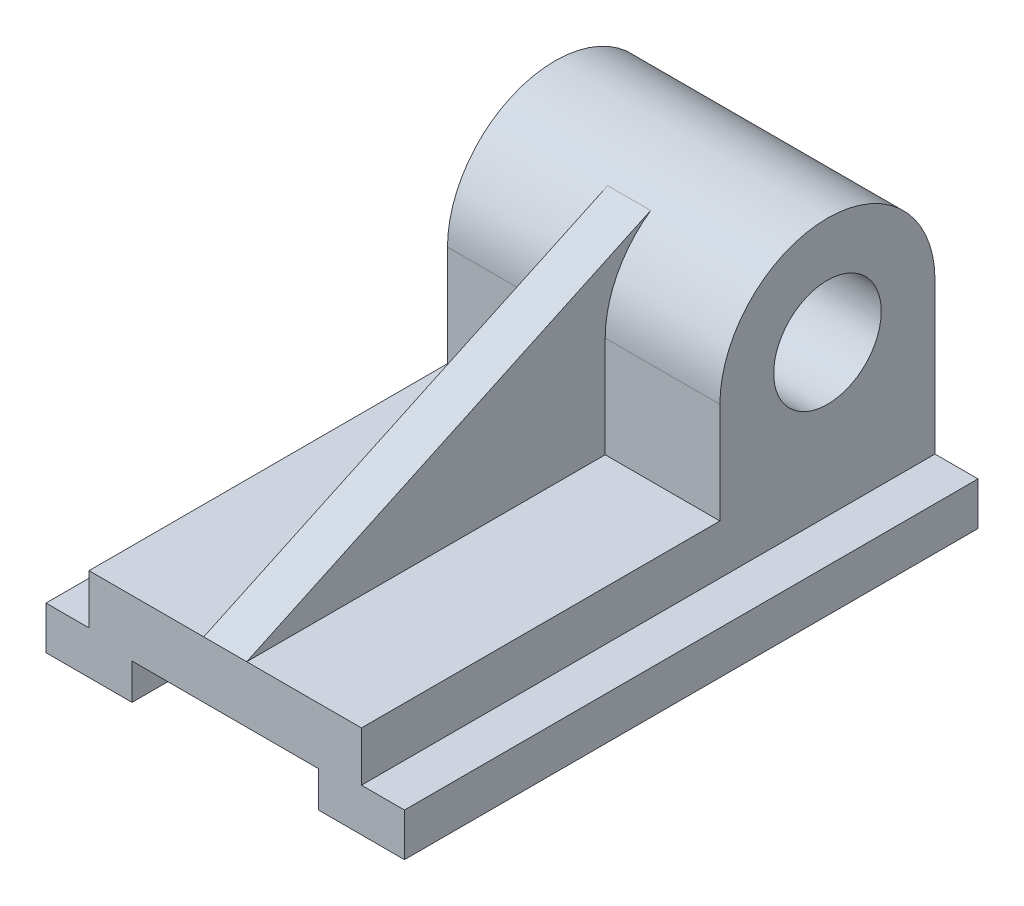
ISO-10303-21;
HEADER;
FILE_DESCRIPTION(('STEP AP214'),'2;1');
FILE_NAME('part.step','',(''),(''),'','','');
FILE_SCHEMA(('AUTOMOTIVE_DESIGN { 1 0 10303 214 1 1 1 1 }'));
ENDSEC;
DATA;
#1=APPLICATION_CONTEXT('core data for automotive mechanical design processes');
#2=APPLICATION_PROTOCOL_DEFINITION('international standard','automotive_design',2000,#1);
#3=PRODUCT_CONTEXT('',#1,'mechanical');
#4=PRODUCT('Part','Part','',(#3));
#5=PRODUCT_RELATED_PRODUCT_CATEGORY('part','',(#4));
#6=PRODUCT_DEFINITION_FORMATION('','',#4);
#7=PRODUCT_DEFINITION_CONTEXT('part definition',#1,'design');
#8=PRODUCT_DEFINITION('design','',#6,#7);
#9=PRODUCT_DEFINITION_SHAPE('','',#8);
#10=(LENGTH_UNIT() NAMED_UNIT(*) SI_UNIT(.MILLI.,.METRE.));
#11=(NAMED_UNIT(*) PLANE_ANGLE_UNIT() SI_UNIT($,.RADIAN.));
#12=(NAMED_UNIT(*) SI_UNIT($,.STERADIAN.) SOLID_ANGLE_UNIT());
#13=UNCERTAINTY_MEASURE_WITH_UNIT(LENGTH_MEASURE(1.E-05),#10,'distance_accuracy_value','');
#14=(GEOMETRIC_REPRESENTATION_CONTEXT(3) GLOBAL_UNCERTAINTY_ASSIGNED_CONTEXT((#13)) GLOBAL_UNIT_ASSIGNED_CONTEXT((#10,
#11,#12)) REPRESENTATION_CONTEXT('',''));
#15=CARTESIAN_POINT('',(0.,0.,0.));
#16=DIRECTION('',(0.,0.,1.));
#17=DIRECTION('',(1.,0.,0.));
#18=AXIS2_PLACEMENT_3D('',#15,#16,#17);
#19=CARTESIAN_POINT('',(-50.,44.,30.));
#20=DIRECTION('',(1.,0.,0.));
#21=DIRECTION('',(0.,0.,-1.));
#22=AXIS2_PLACEMENT_3D('',#19,#20,#21);
#23=CYLINDRICAL_SURFACE('',#22,30.);
#24=DIRECTION('',(-1.,0.,0.));
#25=VECTOR('',#24,1.);
#26=CARTESIAN_POINT('',(6.,68.5011775972043,47.3116231575856));
#27=LINE('',#26,#25);
#28=CARTESIAN_POINT('',(6.,68.5011775972043,47.3116231575856));
#29=VERTEX_POINT('',#28);
#30=CARTESIAN_POINT('',(-6.,68.5011775972043,47.3116231575856));
#31=VERTEX_POINT('',#30);
#32=EDGE_CURVE('E324',#29,#31,#27,.T.);
#33=ORIENTED_EDGE('',*,*,#32,.F.);
#34=CARTESIAN_POINT('',(6.,43.9999999999999,29.9999999999998));
#35=DIRECTION('',(-1.,0.,0.));
#36=DIRECTION('',(0.,0.,1.));
#37=AXIS2_PLACEMENT_3D('',#34,#35,#36);
#38=CIRCLE('',#37,30.0000000000002);
#39=CARTESIAN_POINT('',(6.,44.,60.));
#40=VERTEX_POINT('',#39);
#41=EDGE_CURVE('E191',#40,#29,#38,.T.);
#42=ORIENTED_EDGE('',*,*,#41,.F.);
#43=DIRECTION('',(1.,0.,0.));
#44=VECTOR('',#43,1.);
#45=CARTESIAN_POINT('',(-50.,44.,60.));
#46=LINE('',#45,#44);
#47=CARTESIAN_POINT('',(38.,44.,60.));
#48=VERTEX_POINT('',#47);
#49=EDGE_CURVE('E188',#40,#48,#46,.T.);
#50=ORIENTED_EDGE('',*,*,#49,.T.);
#51=CARTESIAN_POINT('',(38.,44.,30.));
#52=DIRECTION('',(1.,0.,0.));
#53=DIRECTION('',(0.,0.,-1.));
#54=AXIS2_PLACEMENT_3D('',#51,#52,#53);
#55=CIRCLE('',#54,30.);
#56=CARTESIAN_POINT('',(38.,44.,0.));
#57=VERTEX_POINT('',#56);
#58=EDGE_CURVE('E302',#57,#48,#55,.T.);
#59=ORIENTED_EDGE('',*,*,#58,.F.);
#60=DIRECTION('',(1.,0.,0.));
#61=VECTOR('',#60,1.);
#62=CARTESIAN_POINT('',(-50.,44.,0.));
#63=LINE('',#62,#61);
#64=CARTESIAN_POINT('',(-38.,44.,0.));
#65=VERTEX_POINT('',#64);
#66=EDGE_CURVE('E11',#65,#57,#63,.T.);
#67=ORIENTED_EDGE('',*,*,#66,.F.);
#68=CARTESIAN_POINT('',(-38.,44.,30.));
#69=DIRECTION('',(-1.,0.,0.));
#70=DIRECTION('',(0.,0.,1.));
#71=AXIS2_PLACEMENT_3D('',#68,#69,#70);
#72=CIRCLE('',#71,30.);
#73=CARTESIAN_POINT('',(-38.,44.,60.));
#74=VERTEX_POINT('',#73);
#75=EDGE_CURVE('E55',#74,#65,#72,.T.);
#76=ORIENTED_EDGE('',*,*,#75,.F.);
#77=CARTESIAN_POINT('',(-6.,44.,60.));
#78=VERTEX_POINT('',#77);
#79=EDGE_CURVE('E204',#74,#78,#46,.T.);
#80=ORIENTED_EDGE('',*,*,#79,.T.);
#81=CARTESIAN_POINT('',(-6.,43.9999999999999,29.9999999999998));
#82=DIRECTION('',(-1.,0.,0.));
#83=DIRECTION('',(0.,0.,1.));
#84=AXIS2_PLACEMENT_3D('',#81,#82,#83);
#85=CIRCLE('',#84,30.0000000000002);
#86=EDGE_CURVE('E335',#78,#31,#85,.T.);
#87=ORIENTED_EDGE('',*,*,#86,.T.);
#88=EDGE_LOOP('',(#33,#42,#50,#59,#67,#76,#80,#87));
#89=FACE_BOUND('',#88,.T.);
#90=ADVANCED_FACE('F43',(#89),#23,.T.);
#91=CARTESIAN_POINT('',(-50.,0.,60.));
#92=DIRECTION('',(0.,0.,1.));
#93=DIRECTION('',(1.,0.,0.));
#94=AXIS2_PLACEMENT_3D('',#91,#92,#93);
#95=PLANE('',#94);
#96=ORIENTED_EDGE('',*,*,#49,.F.);
#97=DIRECTION('',(0.,1.,0.));
#98=VECTOR('',#97,1.);
#99=CARTESIAN_POINT('',(6.,15.8288601385803,60.));
#100=LINE('',#99,#98);
#101=CARTESIAN_POINT('',(6.,15.8288601385803,60.));
#102=VERTEX_POINT('',#101);
#103=EDGE_CURVE('E171',#102,#40,#100,.T.);
#104=ORIENTED_EDGE('',*,*,#103,.F.);
#105=DIRECTION('',(1.,0.,0.));
#106=VECTOR('',#105,1.);
#107=CARTESIAN_POINT('',(-50.,15.8288601385803,60.));
#108=LINE('',#107,#106);
#109=CARTESIAN_POINT('',(38.,15.8288601385803,60.));
#110=VERTEX_POINT('',#109);
#111=EDGE_CURVE('E190',#102,#110,#108,.T.);
#112=ORIENTED_EDGE('',*,*,#111,.T.);
#113=DIRECTION('',(0.,-1.,0.));
#114=VECTOR('',#113,1.);
#115=CARTESIAN_POINT('',(38.,0.,60.));
#116=LINE('',#115,#114);
#117=EDGE_CURVE('E196',#48,#110,#116,.T.);
#118=ORIENTED_EDGE('',*,*,#117,.F.);
#119=EDGE_LOOP('',(#96,#104,#112,#118));
#120=FACE_BOUND('',#119,.T.);
#121=ADVANCED_FACE('F187',(#120),#95,.T.);
#122=CARTESIAN_POINT('',(-50.,15.8288601385803,0.));
#123=DIRECTION('',(0.,-1.,0.));
#124=DIRECTION('',(0.,0.,-1.));
#125=AXIS2_PLACEMENT_3D('',#122,#123,#124);
#126=PLANE('',#125);
#127=DIRECTION('',(0.,0.,-1.));
#128=VECTOR('',#127,1.);
#129=CARTESIAN_POINT('',(6.,15.8288601385803,160.));
#130=LINE('',#129,#128);
#131=CARTESIAN_POINT('',(6.,15.8288601385803,160.));
#132=VERTEX_POINT('',#131);
#133=EDGE_CURVE('E172',#132,#102,#130,.T.);
#134=ORIENTED_EDGE('',*,*,#133,.F.);
#135=DIRECTION('',(1.,0.,0.));
#136=VECTOR('',#135,1.);
#137=CARTESIAN_POINT('',(0.,15.8288601385803,160.));
#138=LINE('',#137,#136);
#139=CARTESIAN_POINT('',(38.,15.8288601385803,160.));
#140=VERTEX_POINT('',#139);
#141=EDGE_CURVE('E287',#132,#140,#138,.T.);
#142=ORIENTED_EDGE('',*,*,#141,.T.);
#143=DIRECTION('',(0.,0.,-1.));
#144=VECTOR('',#143,1.);
#145=CARTESIAN_POINT('',(38.,15.8288601385803,0.));
#146=LINE('',#145,#144);
#147=EDGE_CURVE('E195',#140,#110,#146,.T.);
#148=ORIENTED_EDGE('',*,*,#147,.T.);
#149=ORIENTED_EDGE('',*,*,#111,.F.);
#150=EDGE_LOOP('',(#134,#142,#148,#149));
#151=FACE_BOUND('',#150,.T.);
#152=ADVANCED_FACE('F194',(#151),#126,.F.);
#153=CARTESIAN_POINT('',(38.,0.,160.));
#154=DIRECTION('',(-1.,0.,0.));
#155=DIRECTION('',(0.,0.,1.));
#156=AXIS2_PLACEMENT_3D('',#153,#154,#155);
#157=PLANE('',#156);
#158=CARTESIAN_POINT('',(38.,44.,30.));
#159=DIRECTION('',(1.,0.,0.));
#160=DIRECTION('',(0.,0.,-1.));
#161=AXIS2_PLACEMENT_3D('',#158,#159,#160);
#162=CIRCLE('',#161,15.);
#163=CARTESIAN_POINT('',(38.,44.,15.));
#164=VERTEX_POINT('',#163);
#165=EDGE_CURVE('E339',#164,#164,#162,.T.);
#166=ORIENTED_EDGE('',*,*,#165,.F.);
#167=EDGE_LOOP('',(#166));
#168=FACE_BOUND('',#167,.T.);
#169=DIRECTION('',(0.,1.,0.));
#170=VECTOR('',#169,1.);
#171=CARTESIAN_POINT('',(38.,0.,0.));
#172=LINE('',#171,#170);
#173=CARTESIAN_POINT('',(38.,2.,0.));
#174=VERTEX_POINT('',#173);
#175=EDGE_CURVE('E206',#174,#57,#172,.T.);
#176=ORIENTED_EDGE('',*,*,#175,.T.);
#177=ORIENTED_EDGE('',*,*,#58,.T.);
#178=ORIENTED_EDGE('',*,*,#117,.T.);
#179=ORIENTED_EDGE('',*,*,#147,.F.);
#180=DIRECTION('',(0.,1.,0.));
#181=VECTOR('',#180,1.);
#182=CARTESIAN_POINT('',(38.,0.,160.));
#183=LINE('',#182,#181);
#184=CARTESIAN_POINT('',(38.,2.,160.));
#185=VERTEX_POINT('',#184);
#186=EDGE_CURVE('E210',#185,#140,#183,.T.);
#187=ORIENTED_EDGE('',*,*,#186,.F.);
#188=DIRECTION('',(0.,0.,-1.));
#189=VECTOR('',#188,1.);
#190=CARTESIAN_POINT('',(38.,2.,160.));
#191=LINE('',#190,#189);
#192=EDGE_CURVE('E237',#185,#174,#191,.T.);
#193=ORIENTED_EDGE('',*,*,#192,.T.);
#194=EDGE_LOOP('',(#176,#177,#178,#179,#187,#193));
#195=FACE_BOUND('',#194,.T.);
#196=ADVANCED_FACE('F44',(#168,#195),#157,.F.);
#197=CARTESIAN_POINT('',(-38.,0.,160.));
#198=DIRECTION('',(-1.,0.,0.));
#199=DIRECTION('',(0.,0.,1.));
#200=AXIS2_PLACEMENT_3D('',#197,#198,#199);
#201=PLANE('',#200);
#202=CARTESIAN_POINT('',(-38.,44.,30.));
#203=DIRECTION('',(-1.,0.,0.));
#204=DIRECTION('',(0.,0.,1.));
#205=AXIS2_PLACEMENT_3D('',#202,#203,#204);
#206=CIRCLE('',#205,15.);
#207=CARTESIAN_POINT('',(-38.,44.,45.));
#208=VERTEX_POINT('',#207);
#209=EDGE_CURVE('E50',#208,#208,#206,.T.);
#210=ORIENTED_EDGE('',*,*,#209,.F.);
#211=EDGE_LOOP('',(#210));
#212=FACE_BOUND('',#211,.T.);
#213=ORIENTED_EDGE('',*,*,#75,.T.);
#214=DIRECTION('',(0.,1.,0.));
#215=VECTOR('',#214,1.);
#216=CARTESIAN_POINT('',(-38.,0.,0.));
#217=LINE('',#216,#215);
#218=CARTESIAN_POINT('',(-38.,2.,0.));
#219=VERTEX_POINT('',#218);
#220=EDGE_CURVE('E239',#219,#65,#217,.T.);
#221=ORIENTED_EDGE('',*,*,#220,.F.);
#222=DIRECTION('',(0.,0.,-1.));
#223=VECTOR('',#222,1.);
#224=CARTESIAN_POINT('',(-38.,2.,160.));
#225=LINE('',#224,#223);
#226=CARTESIAN_POINT('',(-38.,2.,160.));
#227=VERTEX_POINT('',#226);
#228=EDGE_CURVE('E283',#227,#219,#225,.T.);
#229=ORIENTED_EDGE('',*,*,#228,.F.);
#230=DIRECTION('',(0.,1.,0.));
#231=VECTOR('',#230,1.);
#232=CARTESIAN_POINT('',(-38.,0.,160.));
#233=LINE('',#232,#231);
#234=CARTESIAN_POINT('',(-38.,15.8288601385803,160.));
#235=VERTEX_POINT('',#234);
#236=EDGE_CURVE('E209',#227,#235,#233,.T.);
#237=ORIENTED_EDGE('',*,*,#236,.T.);
#238=DIRECTION('',(0.,0.,1.));
#239=VECTOR('',#238,1.);
#240=CARTESIAN_POINT('',(-38.,15.8288601385803,160.));
#241=LINE('',#240,#239);
#242=CARTESIAN_POINT('',(-38.,15.8288601385803,60.));
#243=VERTEX_POINT('',#242);
#244=EDGE_CURVE('E67',#243,#235,#241,.T.);
#245=ORIENTED_EDGE('',*,*,#244,.F.);
#246=DIRECTION('',(0.,1.,0.));
#247=VECTOR('',#246,1.);
#248=CARTESIAN_POINT('',(-38.,0.,60.));
#249=LINE('',#248,#247);
#250=EDGE_CURVE('E290',#243,#74,#249,.T.);
#251=ORIENTED_EDGE('',*,*,#250,.T.);
#252=EDGE_LOOP('',(#213,#221,#229,#237,#245,#251));
#253=FACE_BOUND('',#252,.T.);
#254=ADVANCED_FACE('F297',(#212,#253),#201,.T.);
#255=CARTESIAN_POINT('',(0.,2.,160.));
#256=DIRECTION('',(0.,1.,0.));
#257=DIRECTION('',(0.,0.,1.));
#258=AXIS2_PLACEMENT_3D('',#255,#256,#257);
#259=PLANE('',#258);
#260=DIRECTION('',(1.,0.,0.));
#261=VECTOR('',#260,1.);
#262=CARTESIAN_POINT('',(0.,2.,0.));
#263=LINE('',#262,#261);
#264=CARTESIAN_POINT('',(-50.,2.,0.));
#265=VERTEX_POINT('',#264);
#266=EDGE_CURVE('E244',#265,#219,#263,.T.);
#267=ORIENTED_EDGE('',*,*,#266,.F.);
#268=DIRECTION('',(0.,0.,-1.));
#269=VECTOR('',#268,1.);
#270=CARTESIAN_POINT('',(-50.,2.,160.));
#271=LINE('',#270,#269);
#272=CARTESIAN_POINT('',(-50.,2.,160.));
#273=VERTEX_POINT('',#272);
#274=EDGE_CURVE('E285',#273,#265,#271,.T.);
#275=ORIENTED_EDGE('',*,*,#274,.F.);
#276=DIRECTION('',(1.,0.,0.));
#277=VECTOR('',#276,1.);
#278=CARTESIAN_POINT('',(0.,2.,160.));
#279=LINE('',#278,#277);
#280=EDGE_CURVE('E212',#273,#227,#279,.T.);
#281=ORIENTED_EDGE('',*,*,#280,.T.);
#282=ORIENTED_EDGE('',*,*,#228,.T.);
#283=EDGE_LOOP('',(#267,#275,#281,#282));
#284=FACE_BOUND('',#283,.T.);
#285=ADVANCED_FACE('F310',(#284),#259,.T.);
#286=CARTESIAN_POINT('',(-50.,0.,160.));
#287=DIRECTION('',(-1.,0.,0.));
#288=DIRECTION('',(0.,0.,1.));
#289=AXIS2_PLACEMENT_3D('',#286,#287,#288);
#290=PLANE('',#289);
#291=DIRECTION('',(0.,1.,0.));
#292=VECTOR('',#291,1.);
#293=CARTESIAN_POINT('',(-50.,0.,0.));
#294=LINE('',#293,#292);
#295=CARTESIAN_POINT('',(-50.,-10.,0.));
#296=VERTEX_POINT('',#295);
#297=EDGE_CURVE('E243',#296,#265,#294,.T.);
#298=ORIENTED_EDGE('',*,*,#297,.F.);
#299=DIRECTION('',(0.,0.,-1.));
#300=VECTOR('',#299,1.);
#301=CARTESIAN_POINT('',(-50.,-10.,160.));
#302=LINE('',#301,#300);
#303=CARTESIAN_POINT('',(-50.,-10.,160.));
#304=VERTEX_POINT('',#303);
#305=EDGE_CURVE('E282',#304,#296,#302,.T.);
#306=ORIENTED_EDGE('',*,*,#305,.F.);
#307=DIRECTION('',(0.,1.,0.));
#308=VECTOR('',#307,1.);
#309=CARTESIAN_POINT('',(-50.,0.,160.));
#310=LINE('',#309,#308);
#311=EDGE_CURVE('E220',#304,#273,#310,.T.);
#312=ORIENTED_EDGE('',*,*,#311,.T.);
#313=ORIENTED_EDGE('',*,*,#274,.T.);
#314=EDGE_LOOP('',(#298,#306,#312,#313));
#315=FACE_BOUND('',#314,.T.);
#316=ADVANCED_FACE('F354',(#315),#290,.T.);
#317=CARTESIAN_POINT('',(0.,-10.,160.));
#318=DIRECTION('',(0.,-1.,0.));
#319=DIRECTION('',(1.,0.,0.));
#320=AXIS2_PLACEMENT_3D('',#317,#318,#319);
#321=PLANE('',#320);
#322=DIRECTION('',(-1.,0.,0.));
#323=VECTOR('',#322,1.);
#324=CARTESIAN_POINT('',(0.,-10.,0.));
#325=LINE('',#324,#323);
#326=CARTESIAN_POINT('',(-26.,-10.,0.));
#327=VERTEX_POINT('',#326);
#328=EDGE_CURVE('E249',#327,#296,#325,.T.);
#329=ORIENTED_EDGE('',*,*,#328,.F.);
#330=DIRECTION('',(0.,0.,-1.));
#331=VECTOR('',#330,1.);
#332=CARTESIAN_POINT('',(-26.,-10.,160.));
#333=LINE('',#332,#331);
#334=CARTESIAN_POINT('',(-26.,-10.,160.));
#335=VERTEX_POINT('',#334);
#336=EDGE_CURVE('E276',#335,#327,#333,.T.);
#337=ORIENTED_EDGE('',*,*,#336,.F.);
#338=DIRECTION('',(-1.,0.,0.));
#339=VECTOR('',#338,1.);
#340=CARTESIAN_POINT('',(0.,-10.,160.));
#341=LINE('',#340,#339);
#342=EDGE_CURVE('E219',#335,#304,#341,.T.);
#343=ORIENTED_EDGE('',*,*,#342,.T.);
#344=ORIENTED_EDGE('',*,*,#305,.T.);
#345=EDGE_LOOP('',(#329,#337,#343,#344));
#346=FACE_BOUND('',#345,.T.);
#347=ADVANCED_FACE('F388',(#346),#321,.T.);
#348=CARTESIAN_POINT('',(-26.,0.,160.));
#349=DIRECTION('',(1.,0.,0.));
#350=DIRECTION('',(0.,0.,-1.));
#351=AXIS2_PLACEMENT_3D('',#348,#349,#350);
#352=PLANE('',#351);
#353=DIRECTION('',(0.,-1.,0.));
#354=VECTOR('',#353,1.);
#355=CARTESIAN_POINT('',(-26.,0.,0.));
#356=LINE('',#355,#354);
#357=CARTESIAN_POINT('',(-26.,0.,0.));
#358=VERTEX_POINT('',#357);
#359=EDGE_CURVE('E253',#358,#327,#356,.T.);
#360=ORIENTED_EDGE('',*,*,#359,.F.);
#361=DIRECTION('',(0.,0.,-1.));
#362=VECTOR('',#361,1.);
#363=CARTESIAN_POINT('',(-26.,0.,160.));
#364=LINE('',#363,#362);
#365=CARTESIAN_POINT('',(-26.,0.,160.));
#366=VERTEX_POINT('',#365);
#367=EDGE_CURVE('E280',#366,#358,#364,.T.);
#368=ORIENTED_EDGE('',*,*,#367,.F.);
#369=DIRECTION('',(0.,-1.,0.));
#370=VECTOR('',#369,1.);
#371=CARTESIAN_POINT('',(-26.,0.,160.));
#372=LINE('',#371,#370);
#373=EDGE_CURVE('E224',#366,#335,#372,.T.);
#374=ORIENTED_EDGE('',*,*,#373,.T.);
#375=ORIENTED_EDGE('',*,*,#336,.T.);
#376=EDGE_LOOP('',(#360,#368,#374,#375));
#377=FACE_BOUND('',#376,.T.);
#378=ADVANCED_FACE('F387',(#377),#352,.T.);
#379=CARTESIAN_POINT('',(0.,0.,160.));
#380=DIRECTION('',(0.,1.,0.));
#381=DIRECTION('',(0.,0.,1.));
#382=AXIS2_PLACEMENT_3D('',#379,#380,#381);
#383=PLANE('',#382);
#384=DIRECTION('',(1.,0.,0.));
#385=VECTOR('',#384,1.);
#386=CARTESIAN_POINT('',(0.,0.,0.));
#387=LINE('',#386,#385);
#388=CARTESIAN_POINT('',(26.,0.,0.));
#389=VERTEX_POINT('',#388);
#390=EDGE_CURVE('E255',#358,#389,#387,.T.);
#391=ORIENTED_EDGE('',*,*,#390,.T.);
#392=DIRECTION('',(0.,0.,-1.));
#393=VECTOR('',#392,1.);
#394=CARTESIAN_POINT('',(26.,0.,160.));
#395=LINE('',#394,#393);
#396=CARTESIAN_POINT('',(26.,0.,160.));
#397=VERTEX_POINT('',#396);
#398=EDGE_CURVE('E273',#397,#389,#395,.T.);
#399=ORIENTED_EDGE('',*,*,#398,.F.);
#400=DIRECTION('',(1.,0.,0.));
#401=VECTOR('',#400,1.);
#402=CARTESIAN_POINT('',(0.,0.,160.));
#403=LINE('',#402,#401);
#404=EDGE_CURVE('E227',#366,#397,#403,.T.);
#405=ORIENTED_EDGE('',*,*,#404,.F.);
#406=ORIENTED_EDGE('',*,*,#367,.T.);
#407=EDGE_LOOP('',(#391,#399,#405,#406));
#408=FACE_BOUND('',#407,.T.);
#409=ADVANCED_FACE('F385',(#408),#383,.F.);
#410=CARTESIAN_POINT('',(26.,0.,160.));
#411=DIRECTION('',(1.,0.,0.));
#412=DIRECTION('',(0.,1.,0.));
#413=AXIS2_PLACEMENT_3D('',#410,#411,#412);
#414=PLANE('',#413);
#415=DIRECTION('',(0.,-1.,0.));
#416=VECTOR('',#415,1.);
#417=CARTESIAN_POINT('',(26.,0.,0.));
#418=LINE('',#417,#416);
#419=CARTESIAN_POINT('',(26.,-10.,0.));
#420=VERTEX_POINT('',#419);
#421=EDGE_CURVE('E258',#389,#420,#418,.T.);
#422=ORIENTED_EDGE('',*,*,#421,.T.);
#423=DIRECTION('',(0.,0.,-1.));
#424=VECTOR('',#423,1.);
#425=CARTESIAN_POINT('',(26.,-10.,160.));
#426=LINE('',#425,#424);
#427=CARTESIAN_POINT('',(26.,-10.,160.));
#428=VERTEX_POINT('',#427);
#429=EDGE_CURVE('E271',#428,#420,#426,.T.);
#430=ORIENTED_EDGE('',*,*,#429,.F.);
#431=DIRECTION('',(0.,-1.,0.));
#432=VECTOR('',#431,1.);
#433=CARTESIAN_POINT('',(26.,0.,160.));
#434=LINE('',#433,#432);
#435=EDGE_CURVE('E230',#397,#428,#434,.T.);
#436=ORIENTED_EDGE('',*,*,#435,.F.);
#437=ORIENTED_EDGE('',*,*,#398,.T.);
#438=EDGE_LOOP('',(#422,#430,#436,#437));
#439=FACE_BOUND('',#438,.T.);
#440=ADVANCED_FACE('F378',(#439),#414,.F.);
#441=CARTESIAN_POINT('',(0.,-10.,160.));
#442=DIRECTION('',(0.,1.,0.));
#443=DIRECTION('',(-1.,0.,0.));
#444=AXIS2_PLACEMENT_3D('',#441,#442,#443);
#445=PLANE('',#444);
#446=DIRECTION('',(1.,0.,0.));
#447=VECTOR('',#446,1.);
#448=CARTESIAN_POINT('',(0.,-10.,0.));
#449=LINE('',#448,#447);
#450=CARTESIAN_POINT('',(50.,-10.,0.));
#451=VERTEX_POINT('',#450);
#452=EDGE_CURVE('E256',#420,#451,#449,.T.);
#453=ORIENTED_EDGE('',*,*,#452,.T.);
#454=DIRECTION('',(0.,0.,-1.));
#455=VECTOR('',#454,1.);
#456=CARTESIAN_POINT('',(50.,-10.,160.));
#457=LINE('',#456,#455);
#458=CARTESIAN_POINT('',(50.,-10.,160.));
#459=VERTEX_POINT('',#458);
#460=EDGE_CURVE('E268',#459,#451,#457,.T.);
#461=ORIENTED_EDGE('',*,*,#460,.F.);
#462=DIRECTION('',(1.,0.,0.));
#463=VECTOR('',#462,1.);
#464=CARTESIAN_POINT('',(0.,-10.,160.));
#465=LINE('',#464,#463);
#466=EDGE_CURVE('E228',#428,#459,#465,.T.);
#467=ORIENTED_EDGE('',*,*,#466,.F.);
#468=ORIENTED_EDGE('',*,*,#429,.T.);
#469=EDGE_LOOP('',(#453,#461,#467,#468));
#470=FACE_BOUND('',#469,.T.);
#471=ADVANCED_FACE('F372',(#470),#445,.F.);
#472=CARTESIAN_POINT('',(50.,0.,160.));
#473=DIRECTION('',(-1.,0.,0.));
#474=DIRECTION('',(0.,0.,1.));
#475=AXIS2_PLACEMENT_3D('',#472,#473,#474);
#476=PLANE('',#475);
#477=DIRECTION('',(0.,1.,0.));
#478=VECTOR('',#477,1.);
#479=CARTESIAN_POINT('',(50.,0.,0.));
#480=LINE('',#479,#478);
#481=CARTESIAN_POINT('',(50.,2.,0.));
#482=VERTEX_POINT('',#481);
#483=EDGE_CURVE('E257',#451,#482,#480,.T.);
#484=ORIENTED_EDGE('',*,*,#483,.T.);
#485=DIRECTION('',(0.,0.,-1.));
#486=VECTOR('',#485,1.);
#487=CARTESIAN_POINT('',(50.,2.,160.));
#488=LINE('',#487,#486);
#489=CARTESIAN_POINT('',(50.,2.,160.));
#490=VERTEX_POINT('',#489);
#491=EDGE_CURVE('E264',#490,#482,#488,.T.);
#492=ORIENTED_EDGE('',*,*,#491,.F.);
#493=DIRECTION('',(0.,1.,0.));
#494=VECTOR('',#493,1.);
#495=CARTESIAN_POINT('',(50.,0.,160.));
#496=LINE('',#495,#494);
#497=EDGE_CURVE('E232',#459,#490,#496,.T.);
#498=ORIENTED_EDGE('',*,*,#497,.F.);
#499=ORIENTED_EDGE('',*,*,#460,.T.);
#500=EDGE_LOOP('',(#484,#492,#498,#499));
#501=FACE_BOUND('',#500,.T.);
#502=ADVANCED_FACE('F367',(#501),#476,.F.);
#503=CARTESIAN_POINT('',(0.,2.,160.));
#504=DIRECTION('',(0.,-1.,0.));
#505=DIRECTION('',(0.,0.,-1.));
#506=AXIS2_PLACEMENT_3D('',#503,#504,#505);
#507=PLANE('',#506);
#508=DIRECTION('',(-1.,0.,0.));
#509=VECTOR('',#508,1.);
#510=CARTESIAN_POINT('',(0.,2.,0.));
#511=LINE('',#510,#509);
#512=EDGE_CURVE('E211',#482,#174,#511,.T.);
#513=ORIENTED_EDGE('',*,*,#512,.T.);
#514=ORIENTED_EDGE('',*,*,#192,.F.);
#515=DIRECTION('',(-1.,0.,0.));
#516=VECTOR('',#515,1.);
#517=CARTESIAN_POINT('',(0.,2.,160.));
#518=LINE('',#517,#516);
#519=EDGE_CURVE('E233',#490,#185,#518,.T.);
#520=ORIENTED_EDGE('',*,*,#519,.F.);
#521=ORIENTED_EDGE('',*,*,#491,.T.);
#522=EDGE_LOOP('',(#513,#514,#520,#521));
#523=FACE_BOUND('',#522,.T.);
#524=ADVANCED_FACE('F368',(#523),#507,.F.);
#525=CARTESIAN_POINT('',(0.,0.,160.));
#526=DIRECTION('',(0.,0.,1.));
#527=DIRECTION('',(1.,0.,0.));
#528=AXIS2_PLACEMENT_3D('',#525,#526,#527);
#529=PLANE('',#528);
#530=CARTESIAN_POINT('',(-6.,15.8288601385803,160.));
#531=VERTEX_POINT('',#530);
#532=EDGE_CURVE('E289',#235,#531,#138,.T.);
#533=ORIENTED_EDGE('',*,*,#532,.F.);
#534=ORIENTED_EDGE('',*,*,#236,.F.);
#535=ORIENTED_EDGE('',*,*,#280,.F.);
#536=ORIENTED_EDGE('',*,*,#311,.F.);
#537=ORIENTED_EDGE('',*,*,#342,.F.);
#538=ORIENTED_EDGE('',*,*,#373,.F.);
#539=ORIENTED_EDGE('',*,*,#404,.T.);
#540=ORIENTED_EDGE('',*,*,#435,.T.);
#541=ORIENTED_EDGE('',*,*,#466,.T.);
#542=ORIENTED_EDGE('',*,*,#497,.T.);
#543=ORIENTED_EDGE('',*,*,#519,.T.);
#544=ORIENTED_EDGE('',*,*,#186,.T.);
#545=ORIENTED_EDGE('',*,*,#141,.F.);
#546=DIRECTION('',(-1.,0.,0.));
#547=VECTOR('',#546,1.);
#548=CARTESIAN_POINT('',(6.,15.8288601385803,160.));
#549=LINE('',#548,#547);
#550=EDGE_CURVE('E316',#132,#531,#549,.T.);
#551=ORIENTED_EDGE('',*,*,#550,.T.);
#552=EDGE_LOOP('',(#533,#534,#535,#536,#537,#538,#539,#540,#541,#542,#543,#544,#545,#551));
#553=FACE_BOUND('',#552,.T.);
#554=ADVANCED_FACE('F311',(#553),#529,.T.);
#555=CARTESIAN_POINT('',(0.,0.,0.));
#556=DIRECTION('',(0.,0.,1.));
#557=DIRECTION('',(1.,0.,0.));
#558=AXIS2_PLACEMENT_3D('',#555,#556,#557);
#559=PLANE('',#558);
#560=ORIENTED_EDGE('',*,*,#220,.T.);
#561=ORIENTED_EDGE('',*,*,#66,.T.);
#562=ORIENTED_EDGE('',*,*,#175,.F.);
#563=ORIENTED_EDGE('',*,*,#512,.F.);
#564=ORIENTED_EDGE('',*,*,#483,.F.);
#565=ORIENTED_EDGE('',*,*,#452,.F.);
#566=ORIENTED_EDGE('',*,*,#421,.F.);
#567=ORIENTED_EDGE('',*,*,#390,.F.);
#568=ORIENTED_EDGE('',*,*,#359,.T.);
#569=ORIENTED_EDGE('',*,*,#328,.T.);
#570=ORIENTED_EDGE('',*,*,#297,.T.);
#571=ORIENTED_EDGE('',*,*,#266,.T.);
#572=EDGE_LOOP('',(#560,#561,#562,#563,#564,#565,#566,#567,#568,#569,#570,#571));
#573=FACE_BOUND('',#572,.T.);
#574=ADVANCED_FACE('F305',(#573),#559,.F.);
#575=DIRECTION('',(0.,1.,0.));
#576=VECTOR('',#575,1.);
#577=CARTESIAN_POINT('',(-6.,15.8288601385803,60.));
#578=LINE('',#577,#576);
#579=CARTESIAN_POINT('',(-6.,15.8288601385803,60.));
#580=VERTEX_POINT('',#579);
#581=EDGE_CURVE('E56',#580,#78,#578,.T.);
#582=ORIENTED_EDGE('',*,*,#581,.T.);
#583=ORIENTED_EDGE('',*,*,#79,.F.);
#584=ORIENTED_EDGE('',*,*,#250,.F.);
#585=EDGE_CURVE('E197',#243,#580,#108,.T.);
#586=ORIENTED_EDGE('',*,*,#585,.T.);
#587=EDGE_LOOP('',(#582,#583,#584,#586));
#588=FACE_BOUND('',#587,.T.);
#589=ADVANCED_FACE('F325',(#588),#95,.T.);
#590=ORIENTED_EDGE('',*,*,#532,.T.);
#591=DIRECTION('',(0.,0.,-1.));
#592=VECTOR('',#591,1.);
#593=CARTESIAN_POINT('',(-6.,15.8288601385803,160.));
#594=LINE('',#593,#592);
#595=EDGE_CURVE('E318',#531,#580,#594,.T.);
#596=ORIENTED_EDGE('',*,*,#595,.T.);
#597=ORIENTED_EDGE('',*,*,#585,.F.);
#598=ORIENTED_EDGE('',*,*,#244,.T.);
#599=EDGE_LOOP('',(#590,#596,#597,#598));
#600=FACE_BOUND('',#599,.T.);
#601=ADVANCED_FACE('F320',(#600),#126,.F.);
#602=CARTESIAN_POINT('',(6.,15.8288601385803,160.));
#603=DIRECTION('',(0.,-0.905922931257607,-0.423442608415385));
#604=DIRECTION('',(0.,0.423442608415385,-0.905922931257607));
#605=AXIS2_PLACEMENT_3D('',#602,#603,#604);
#606=PLANE('',#605);
#607=DIRECTION('',(0.,-0.423442608415385,0.905922931257607));
#608=VECTOR('',#607,1.);
#609=CARTESIAN_POINT('',(-6.,15.8288601385803,160.));
#610=LINE('',#609,#608);
#611=EDGE_CURVE('E185',#31,#531,#610,.T.);
#612=ORIENTED_EDGE('',*,*,#611,.T.);
#613=ORIENTED_EDGE('',*,*,#550,.F.);
#614=DIRECTION('',(0.,-0.423442608415385,0.905922931257607));
#615=VECTOR('',#614,1.);
#616=CARTESIAN_POINT('',(6.,15.8288601385803,160.));
#617=LINE('',#616,#615);
#618=EDGE_CURVE('E177',#29,#132,#617,.T.);
#619=ORIENTED_EDGE('',*,*,#618,.F.);
#620=ORIENTED_EDGE('',*,*,#32,.T.);
#621=EDGE_LOOP('',(#612,#613,#619,#620));
#622=FACE_BOUND('',#621,.T.);
#623=ADVANCED_FACE('F496',(#622),#606,.F.);
#624=CARTESIAN_POINT('',(6.,43.9999999999999,29.9999999999998));
#625=DIRECTION('',(-1.,0.,0.));
#626=DIRECTION('',(0.,0.,1.));
#627=AXIS2_PLACEMENT_3D('',#624,#625,#626);
#628=PLANE('',#627);
#629=ORIENTED_EDGE('',*,*,#133,.T.);
#630=ORIENTED_EDGE('',*,*,#103,.T.);
#631=ORIENTED_EDGE('',*,*,#41,.T.);
#632=ORIENTED_EDGE('',*,*,#618,.T.);
#633=EDGE_LOOP('',(#629,#630,#631,#632));
#634=FACE_BOUND('',#633,.T.);
#635=ADVANCED_FACE('F175',(#634),#628,.F.);
#636=CARTESIAN_POINT('',(-6.,43.9999999999999,29.9999999999998));
#637=DIRECTION('',(-1.,0.,0.));
#638=DIRECTION('',(0.,0.,1.));
#639=AXIS2_PLACEMENT_3D('',#636,#637,#638);
#640=PLANE('',#639);
#641=ORIENTED_EDGE('',*,*,#595,.F.);
#642=ORIENTED_EDGE('',*,*,#611,.F.);
#643=ORIENTED_EDGE('',*,*,#86,.F.);
#644=ORIENTED_EDGE('',*,*,#581,.F.);
#645=EDGE_LOOP('',(#641,#642,#643,#644));
#646=FACE_BOUND('',#645,.T.);
#647=ADVANCED_FACE('F536',(#646),#640,.T.);
#648=CARTESIAN_POINT('',(-50.,44.,30.));
#649=DIRECTION('',(1.,0.,0.));
#650=DIRECTION('',(0.,0.,-1.));
#651=AXIS2_PLACEMENT_3D('',#648,#649,#650);
#652=CYLINDRICAL_SURFACE('',#651,15.);
#653=ORIENTED_EDGE('',*,*,#209,.T.);
#654=EDGE_LOOP('',(#653));
#655=FACE_BOUND('',#654,.T.);
#656=ORIENTED_EDGE('',*,*,#165,.T.);
#657=EDGE_LOOP('',(#656));
#658=FACE_BOUND('',#657,.T.);
#659=ADVANCED_FACE('F343',(#655,#658),#652,.F.);
#660=CLOSED_SHELL('',(#90,#121,#152,#196,#254,#285,#316,#347,#378,#409,#440,#471,#502,#524,#554,
#574,#589,#601,#623,#635,#647,#659));
#661=MANIFOLD_SOLID_BREP('B2',#660);
#662=ADVANCED_BREP_SHAPE_REPRESENTATION('',(#18,#661),#14);
#663=SHAPE_DEFINITION_REPRESENTATION(#9,#662);
ENDSEC;
END-ISO-10303-21;
